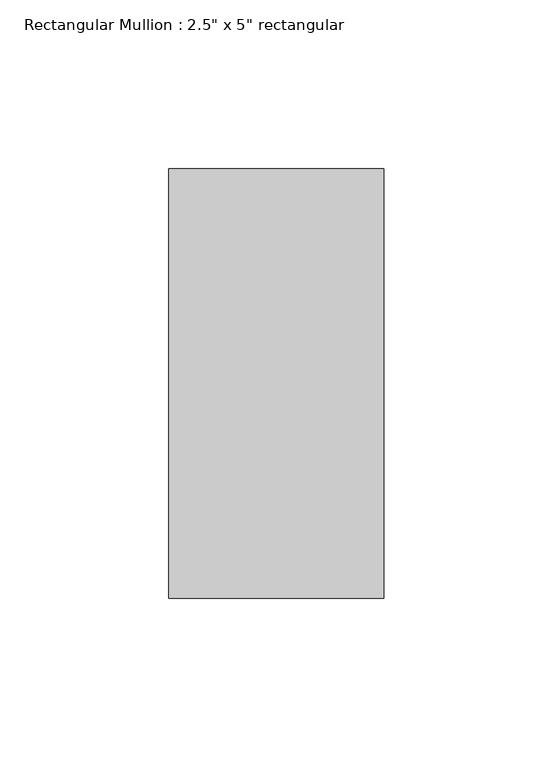
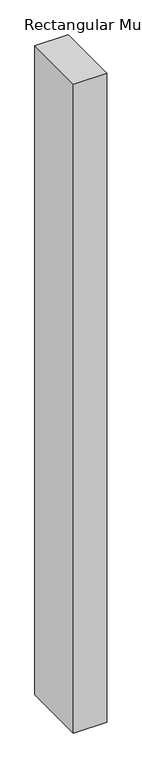
"""IFC4 building model written with IfcOpenShell, lengths in millimetres: member geometry."""

from ifc_helpers import new_model, si_unit, frame, origin, place, context, project, spatial, polyline, outline, extrude, source, transform, mapped, element, save


def member_efb4c79c(model_context):
    return source(origin(), model_context, "Body", "SweptSolid", [
        extrude(outline(polyline([(0.0, 63.5), (0.0, -63.5), (-63.5, -63.5), (-63.5, 63.5), (0.0, 63.5)])), frame((0.0, 0.0, -1305.3654286), z_axis=(0.0, 0.0, 1.0), x_axis=(1.0, 0.0, 0.0)), (0.0, 0.0, 1.0), 1305.3654286),
    ])


if __name__ == "__main__":
    model = new_model("IFC4")
    model_context = context("Model", 3, world=origin())
    ifc_project = project(units=[si_unit("LENGTHUNIT", "METRE", prefix="MILLI")], contexts=[model_context])
    site = spatial("IfcSite", under=ifc_project)
    building = spatial("IfcBuilding", under=site)
    placement = place(None, origin())
    member_shape = member_efb4c79c(model_context)
    element("IfcMember", 1, ObjectType="Rectangular Mullion : 2.5\" x 5\" rectangular", at=placement, inside=building, context=model_context, shape_type="MappedRepresentation", body=[
        mapped(member_shape, transform((0.0, 0.0, 0.0), x_axis=(1.0, 0.0, 0.0), y_axis=(0.0, 1.0, 0.0), z_axis=(0.0, 0.0, 1.0))),
    ])
    save(model, "model.ifc")

# Revit data of these elements
# Type "Rectangular Mullion : 2.5\" x 5\" rectangular"
#   built-in parameter 1007304 = 0.416667 (stored number, unit not read)
#   built-in parameter 1007301 = 0.104167 (stored number, unit not read)
#   built-in parameter 1007300 = 0.104167 (stored number, unit not read)
# Element 1 (IfcMember, "Rectangular Mullion : 2.5\" x 5\" rectangular")
#   Materials on its faces: "Iron, Ductile"
# Materials
#   "Iron, Ductile": class "Metal", colour RGB 0 0 0, transparency 0, Description = "Ductile cast iron", Cost = 0
